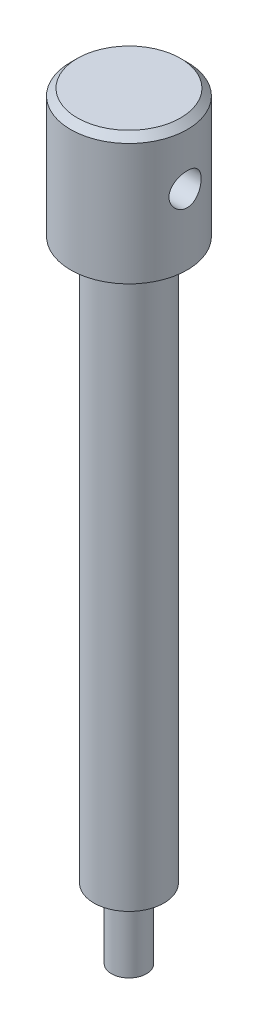
from build123d import *

# Parameters (mm, degrees)
TIP_PIN_SKETCH_6_R        = 3
TIP_PIN_6X12_DEPTH        = 12
SHAFT_SKETCH_12_R         = 6
SHAFT_12X96_DEPTH         = 96
HEAD_SKETCH_20_R          = 10
HEAD_20X22_DEPTH          = 22
CROSS_HOLE_SKETCH_5_5_R   = 2.75
CROSS_HOLE_5_5_DEPTH      = 11
HEAD_CHAMFER_1_15X45_SIZE = 1.15


with BuildPart() as part:
    # Tip Pin Sketch Ø6 → Tip Pin Ø6x12 (new body)
    with BuildSketch(Plane(origin=(0, 0, 0), x_dir=(1, 0, 0), z_dir=(0, 1, 0))):
        with Locations(Location((0, 0, 0), (0, 0, 270))):
            Circle(TIP_PIN_SKETCH_6_R)
    extrude(amount=TIP_PIN_6X12_DEPTH)

    # Shaft Sketch Ø12 → Shaft Ø12x96 (add)
    with BuildSketch(Plane(origin=(0, 12, 0), x_dir=(1, 0, 0), z_dir=(0, 1, 0))):
        with Locations(Location((0, 0, 0), (0, 0, 270))):
            Circle(SHAFT_SKETCH_12_R)
    extrude(amount=SHAFT_12X96_DEPTH)

    # Head Sketch Ø20 → Head Ø20x22 (add)
    with BuildSketch(Plane(origin=(0, 108, 0), x_dir=(1, 0, 0), z_dir=(0, 1, 0))):
        with Locations(Location((0, 0, 0), (0, 0, 270))):
            Circle(HEAD_SKETCH_20_R)
    extrude(amount=HEAD_20X22_DEPTH)

    # Cross Hole Sketch Ø5.5 → Cross Hole Ø5.5 (cut, symmetric)
    with BuildSketch(Plane(origin=(0, 0, 0), x_dir=(0, 0, -1), z_dir=(1, 0, 0))):
        with Locations((0, 120)):
            Circle(CROSS_HOLE_SKETCH_5_5_R)
    extrude(amount=CROSS_HOLE_5_5_DEPTH, both=True, mode=Mode.SUBTRACT)

    # Head Chamfer 1.15x45°
    head_chamfer_1_15x45_edges = [part.edges().sort_by_distance(p)[0] for p in [
        (0, 130, -10),
    ]]
    chamfer(head_chamfer_1_15x45_edges, length=HEAD_CHAMFER_1_15X45_SIZE)


solid = part.part
